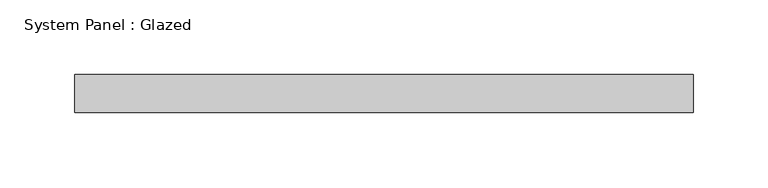
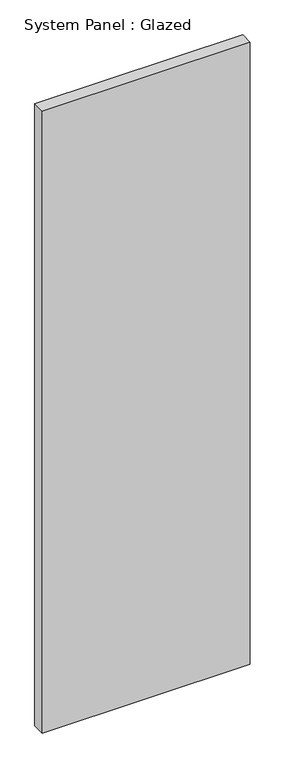
"""IFC4 building model written with IfcOpenShell, lengths in millimetres: plate geometry, System Panel : Glazed."""

from ifc_helpers import new_model, si_unit, origin, origin_with_axes, place, context, project, spatial, polyline, outline, extrude, source, transform, mapped, element, save


def system_panel_glazed_9ae411f7(model_context):
    return source(origin(), model_context, "Body", "SweptSolid", [
        extrude(outline(polyline([(206.375, 19.05), (-206.375, 19.05), (-206.375, 44.45), (206.375, 44.45), (206.375, 19.05)])), origin_with_axes(), (0.0, 0.0, 1.0), 1303.8419021),
    ])


if __name__ == "__main__":
    model = new_model("IFC4")
    model_context = context("Model", 3, world=origin())
    ifc_project = project(units=[si_unit("LENGTHUNIT", "METRE", prefix="MILLI")], contexts=[model_context])
    site = spatial("IfcSite", under=ifc_project)
    building = spatial("IfcBuilding", under=site)
    placement = place(None, origin())
    system_panel_glazed_shape = system_panel_glazed_9ae411f7(model_context)
    element("IfcPlate", 1, ObjectType="System Panel : Glazed", at=placement, inside=building, context=model_context, shape_type="MappedRepresentation", body=[
        mapped(system_panel_glazed_shape, transform((0.0, 0.0, 0.0), x_axis=(1.0, 0.0, 0.0), y_axis=(0.0, 1.0, 0.0), z_axis=(0.0, 0.0, 1.0))),
    ])
    save(model, "model.ifc")

# Revit data of these elements
# Type "System Panel : Glazed"
#   Construction Type Id = "GSP4R"
#   Analytic Construction = "1/8 in Pilkington single glazing"
#   Visual Light Transmittance = 0.9
#   Solar Heat Gain Coefficient = 0.86
#   Heat Transfer Coefficient (U) = 1.18115 BTU/(h·ft²·°F)
#   Define Thermal Properties by = 1
# Element 1 (IfcPlate, "System Panel : Glazed")
#   Materials on its faces: "Glass"
# Materials
#   "Glass": class "Glass", colour RGB 0 128 192, transparency 0.75, Description = "Soda Lime Glass", Cost = 0
